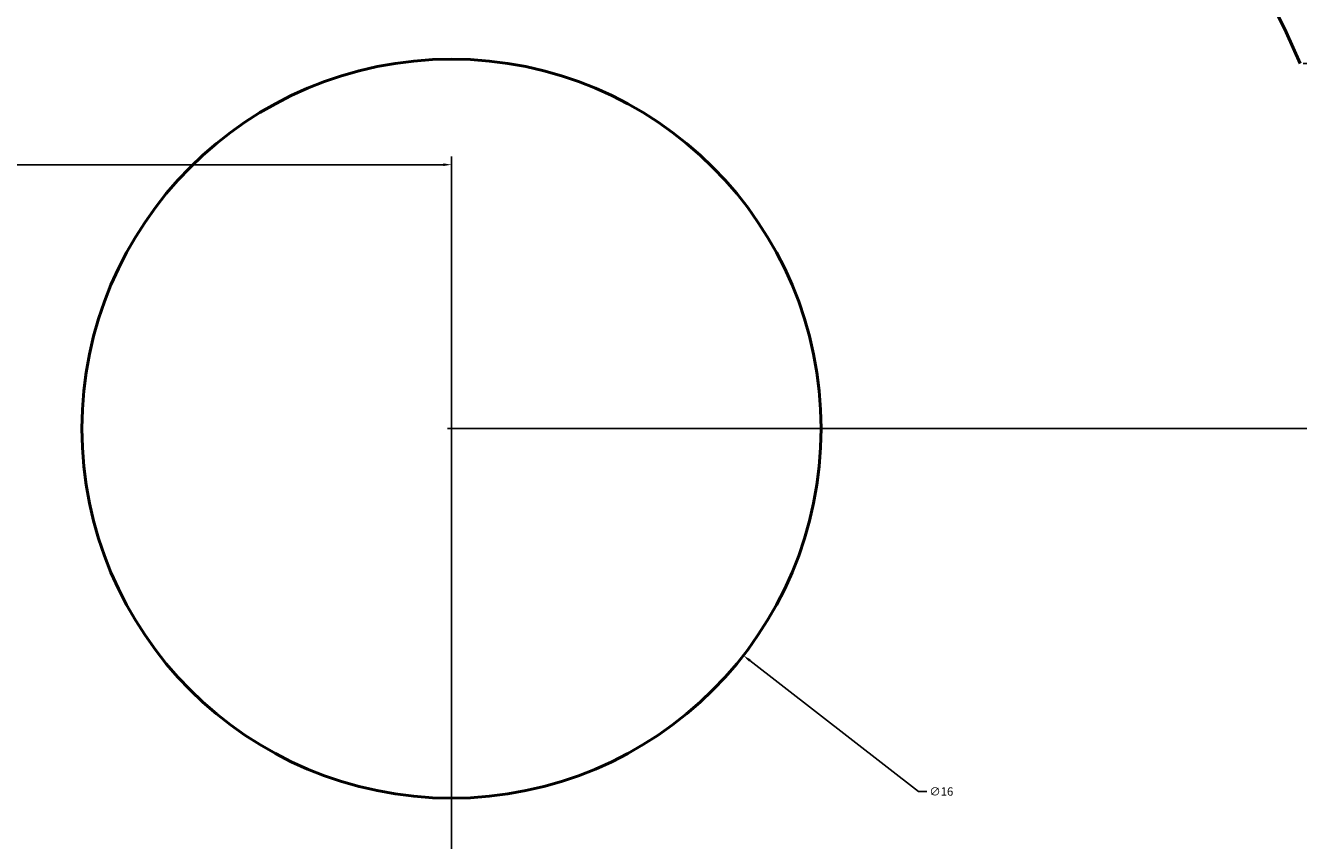
# Model space of a CAD drawing. Units: inches. Extents: x -14 to 108, y -9 to 83.
# Tile 9 of 13: x 38 to 65, y 28 to 46. Entities that reach past the tile are written whole.
import ezdxf

# ---------------------------------------------------------------- set-up
doc = ezdxf.new("R2010")
doc.units = ezdxf.units.IN
doc.header["$MEASUREMENT"] = 0
doc.layers.add('M-DIMS', color=2, linetype='Continuous', lineweight=18)
doc.layers.add('M-OUTL', color=7, linetype='Continuous', lineweight=50)
doc.styles.get("Standard").update_dxf_attribs({"font": 'arial.ttf'})
doc.dimstyles.get("Standard").update_dxf_attribs({"dimtxt": 0.18, "dimasz": 0.18, "dimexe": 0.18, "dimexo": 0.0625, "dimgap": 0.09, "dimtad": 0, "dimtih": 1, "dimtoh": 1, "dimzin": 0, "dimdsep": 46, "dimtxsty": 'Standard', "dimcen": 0.09, "dimadec": 0, "dimazin": 0, "dimtfac": 1, "dimtofl": 0, "dimtmove": 0, "dimatfit": 3, "dimfxl": 1, "dimtolj": 1, "dimtzin": 0, "dimarcsym": 0})

# ---------------------------------------------------------------- blocks, each defined once
blk = doc.blocks.new('*D7')
at = {"layer": 'Defpoints', "color": 0, "transparency": 16777216}
for p in [(47.098, 37.119), (5.951, 18.227), (47.098, -8.596)]:
    blk.add_point(p, dxfattribs=at)
at = {"layer": 'M-DIMS', "color": 0, "lineweight": -2, "transparency": 16777216}
for p, q in [((47.098, 37.057), (47.098, -8.776)), ((5.951, 18.165), (5.951, -8.776)), ((6.131, -8.596), (26.126, -8.596)), ((46.918, -8.596), (26.922, -8.596))]:
    blk.add_line(p, q, dxfattribs=at)
at = {"layer": 'M-DIMS', "color": 0, "transparency": 16777216}
for points in [[(6.131, -8.566), (6.131, -8.626), (5.951, -8.596)], [(46.918, -8.566), (46.918, -8.626), (47.098, -8.596)]]:
    blk.add_solid(points, dxfattribs=at)
at = {"layer": 'M-DIMS', "color": 0, "transparency": 16777216, "insert": (26.524, -8.596), "char_height": 0.18, "attachment_point": 5}
blk.add_mtext('\\A1;41.15', dxfattribs=at)
blk = doc.blocks.new('*D8')
at = {"layer": 'Defpoints', "color": 0, "transparency": 16777216}
for p in [(47.098, 37.119), (81.545, 18.227), (81.545, -8.596)]:
    blk.add_point(p, dxfattribs=at)
at = {"layer": 'M-DIMS', "color": 0, "lineweight": -2, "transparency": 16777216}
for p, q in [((47.098, 37.057), (47.098, -8.776)), ((81.545, 18.165), (81.545, -8.776)), ((47.278, -8.596), (63.927, -8.596)), ((81.365, -8.596), (64.716, -8.596))]:
    blk.add_line(p, q, dxfattribs=at)
at = {"layer": 'M-DIMS', "color": 0, "transparency": 16777216}
for points in [[(47.278, -8.566), (47.278, -8.626), (47.098, -8.596)], [(81.365, -8.566), (81.365, -8.626), (81.545, -8.596)]]:
    blk.add_solid(points, dxfattribs=at)
at = {"layer": 'M-DIMS', "color": 0, "transparency": 16777216, "insert": (64.321, -8.596), "char_height": 0.18, "attachment_point": 5}
blk.add_mtext('\\A1;34.45', dxfattribs=at)
blk = doc.blocks.new('*D11')
at = {"layer": 'Defpoints', "color": 0, "transparency": 16777216}
for p in [(47.098, 37.119), (107.813, 37.119), (86.478, 18.227)]:
    blk.add_point(p, dxfattribs=at)
at = {"layer": 'M-DIMS', "color": 0, "lineweight": -2, "transparency": 16777216}
for p, q in [((47.16, 37.119), (107.993, 37.119)), ((107.813, 36.939), (107.813, 27.855)), ((107.813, 18.407), (107.813, 27.491)), ((86.541, 18.227), (107.993, 18.227))]:
    blk.add_line(p, q, dxfattribs=at)
at = {"layer": 'M-DIMS', "color": 0, "transparency": 16777216}
for points in [[(107.783, 36.939), (107.843, 36.939), (107.813, 37.119)], [(107.783, 18.407), (107.843, 18.407), (107.813, 18.227)]]:
    blk.add_solid(points, dxfattribs=at)
at = {"layer": 'M-DIMS', "color": 0, "transparency": 16777216, "insert": (107.813, 27.673), "char_height": 0.18, "attachment_point": 5}
blk.add_mtext('\\A1;18.892', dxfattribs=at)
blk = doc.blocks.new('*D12')
at = {"layer": 'Defpoints', "color": 0, "transparency": 16777216}
for p in [(86.478, 57.664), (107.813, 57.664), (47.098, 37.119)]:
    blk.add_point(p, dxfattribs=at)
at = {"layer": 'M-DIMS', "color": 0, "lineweight": -2, "transparency": 16777216}
for p, q in [((86.541, 57.664), (107.993, 57.664)), ((107.813, 57.484), (107.813, 47.573)), ((107.813, 37.299), (107.813, 47.21)), ((47.16, 37.119), (107.993, 37.119))]:
    blk.add_line(p, q, dxfattribs=at)
at = {"layer": 'M-DIMS', "color": 0, "transparency": 16777216}
for points in [[(107.783, 57.484), (107.843, 57.484), (107.813, 57.664)], [(107.783, 37.299), (107.843, 37.299), (107.813, 37.119)]]:
    blk.add_solid(points, dxfattribs=at)
at = {"layer": 'M-DIMS', "color": 0, "transparency": 16777216, "insert": (107.813, 47.392), "char_height": 0.18, "attachment_point": 5}
blk.add_mtext('\\A1;20.544', dxfattribs=at)
blk = doc.blocks.new('*D14')
at = {"layer": 'Defpoints', "color": 0, "transparency": 16777216}
for p in [(47.098, 42.834), (16.928, 37.119), (47.098, 37.119)]:
    blk.add_point(p, dxfattribs=at)
at = {"layer": 'M-DIMS', "color": 0, "lineweight": -2, "transparency": 16777216}
for p, q in [((16.928, 37.182), (16.928, 43.014)), ((47.098, 37.182), (47.098, 43.014)), ((17.108, 42.834), (31.619, 42.834)), ((46.918, 42.834), (32.407, 42.834))]:
    blk.add_line(p, q, dxfattribs=at)
at = {"layer": 'M-DIMS', "color": 0, "transparency": 16777216}
for points in [[(17.108, 42.864), (17.108, 42.804), (16.928, 42.834)], [(46.918, 42.864), (46.918, 42.804), (47.098, 42.834)]]:
    blk.add_solid(points, dxfattribs=at)
at = {"layer": 'M-DIMS', "color": 0, "transparency": 16777216, "insert": (32.013, 42.834), "char_height": 0.18, "attachment_point": 5}
blk.add_mtext('\\A1;30.17', dxfattribs=at)
blk = doc.blocks.new('*D21')
at = {"layer": 'Defpoints', "color": 0, "transparency": 16777216}
for p in [(65.47, 45.024), (107.813, 45.024), (47.098, 37.119)]:
    blk.add_point(p, dxfattribs=at)
at = {"layer": 'M-DIMS', "color": 0, "lineweight": -2, "transparency": 16777216}
for p, q in [((65.532, 45.024), (107.993, 45.024)), ((107.813, 44.844), (107.813, 41.254)), ((107.813, 37.299), (107.813, 40.89)), ((47.16, 37.119), (107.993, 37.119))]:
    blk.add_line(p, q, dxfattribs=at)
at = {"layer": 'M-DIMS', "color": 0, "transparency": 16777216}
for points in [[(107.783, 44.844), (107.843, 44.844), (107.813, 45.024)], [(107.783, 37.299), (107.843, 37.299), (107.813, 37.119)]]:
    blk.add_solid(points, dxfattribs=at)
at = {"layer": 'M-DIMS', "color": 0, "transparency": 16777216, "insert": (107.813, 41.072), "char_height": 0.18, "attachment_point": 5}
blk.add_mtext('\\A1;7.905', dxfattribs=at)
blk = doc.blocks.new('*D28')
at = {"layer": 'Defpoints', "color": 0, "transparency": 16777216}
for p in [(40.782, 42.029), (53.414, 32.209)]:
    blk.add_point(p, dxfattribs=at)
at = {"layer": 'M-DIMS', "color": 0, "lineweight": -2, "transparency": 16777216}
for p, q in [((47.098, 37.029), (47.098, 37.209)), ((47.008, 37.119), (47.188, 37.119)), ((57.203, 29.263), (53.556, 32.099)), ((57.383, 29.263), (57.203, 29.263))]:
    blk.add_line(p, q, dxfattribs=at)
at = {"layer": 'M-DIMS', "color": 0, "transparency": 16777216}
blk.add_solid([(53.574, 32.122), (53.538, 32.075), (53.414, 32.209)], dxfattribs=at)
at = {"layer": 'M-DIMS', "color": 0, "transparency": 16777216, "insert": (57.7, 29.263), "char_height": 0.18, "attachment_point": 5}
blk.add_mtext('\\A1;∅16', dxfattribs=at)
blk = doc.blocks.new('*D30')
at = {"layer": 'Defpoints', "color": 0, "transparency": 16777216}
for p in [(59.745, 56.33), (47.098, 37.119)]:
    blk.add_point(p, dxfattribs=at)
at = {"layer": 'M-DIMS', "color": 0, "lineweight": -2, "transparency": 16777216}
for p, q in [((67.333, 67.856), (59.844, 56.48)), ((67.513, 67.856), (67.333, 67.856)), ((47.098, 37.029), (47.098, 37.209)), ((47.008, 37.119), (47.188, 37.119))]:
    blk.add_line(p, q, dxfattribs=at)
at = {"layer": 'M-DIMS', "color": 0, "transparency": 16777216}
blk.add_solid([(59.819, 56.497), (59.869, 56.464), (59.745, 56.33)], dxfattribs=at)
at = {"layer": 'M-DIMS', "color": 0, "transparency": 16777216, "insert": (67.818, 67.856), "char_height": 0.18, "attachment_point": 5}
blk.add_mtext('\\A1;R23', dxfattribs=at)
blk = doc.blocks.new('*D31')
at = {"layer": 'Defpoints', "color": 0, "transparency": 16777216}
for p in [(58.096, 53.824), (47.098, 37.119)]:
    blk.add_point(p, dxfattribs=at)
at = {"layer": 'M-DIMS', "color": 0, "lineweight": -2, "transparency": 16777216}
for p, q in [((64.695, 63.847), (58.195, 53.974)), ((64.875, 63.847), (64.695, 63.847)), ((47.098, 37.029), (47.098, 37.209)), ((47.008, 37.119), (47.188, 37.119))]:
    blk.add_line(p, q, dxfattribs=at)
at = {"layer": 'M-DIMS', "color": 0, "transparency": 16777216}
blk.add_solid([(58.17, 53.991), (58.22, 53.958), (58.096, 53.824)], dxfattribs=at)
at = {"layer": 'M-DIMS', "color": 0, "transparency": 16777216, "insert": (65.18, 63.847), "char_height": 0.18, "attachment_point": 5}
blk.add_mtext('\\A1;R20', dxfattribs=at)

msp = doc.modelspace()

# ---------------------------------------------------------------- linework, layer by layer
at = {"layer": 'M-OUTL'}
msp.add_circle((47.0979, 37.1193), 8, dxfattribs=at)
msp.add_arc((47.0979, 37.1193), 20, 23.2807, 90, dxfattribs=at)

# ---------------------------------------------------------------- dimensions: what is measured, and where the dimension line sits
at = {"layer": 'M-DIMS'}
for mpoint, picture, middle in [((59.745, 56.33), '*D30', (67.8183, 67.8564)), ((58.0959, 53.8239), '*D31', (65.1795, 63.8467))]:
    dim = msp.add_radius_dim(center=(47.0979, 37.1193), mpoint=mpoint, dimstyle='Standard', override={"dimdec": 0, "dimlfac": 1, "dimrnd": 0, "dimzin": 0, "dimdsep": 46, "dimlunit": 2}, dxfattribs=at)
    dim.commit()
    dim.dimension.update_dxf_attribs({"geometry": picture, "text_midpoint": middle, "dimtype": 164})
for base, p1, p2, angle, override, picture, middle in [((107.8129, 57.6637), (47.0979, 37.1193), (86.4784, 57.6637), 90, {"dimdec": 3, "dimlfac": 1, "dimrnd": 0, "dimzin": 0, "dimdsep": 46, "dimlunit": 2}, '*D12', (107.8129, 47.3915)), ((107.8129, 45.0241), (47.0979, 37.1193), (65.4695, 45.0241), 90, {"dimdec": 3, "dimlfac": 1, "dimrnd": 0, "dimzin": 0, "dimdsep": 46, "dimlunit": 2}, '*D21', (107.8129, 41.0717)), ((47.0979, 42.8343), (16.9278, 37.1193), (47.0979, 37.1193), 0, {"dimdec": 2, "dimlfac": 1, "dimrnd": 0, "dimzin": 0, "dimdsep": 46, "dimlunit": 2}, '*D14', (32.0129, 42.8343)), ((107.8129, 37.1193), (86.4784, 18.2274), (47.0979, 37.1193), 90, {"dimdec": 3, "dimlfac": 1, "dimrnd": 0, "dimzin": 0, "dimdsep": 46, "dimlunit": 2}, '*D11', (107.8129, 27.6733))]:
    dim = msp.add_linear_dim(base=base, p1=p1, p2=p2, angle=angle, dimstyle='Standard', override=override, dxfattribs=at)
    dim.commit()
    dim.dimension.update_dxf_attribs({"geometry": picture, "text_midpoint": middle})
dim = msp.add_diameter_dim_2p(p1=(40.782, 42.0294), p2=(53.4138, 32.2092), dimstyle='Standard', override={"dimdec": 0, "dimlfac": 1, "dimrnd": 0, "dimzin": 0, "dimdsep": 46, "dimlunit": 2}, dxfattribs=at)
dim.commit()
dim.dimension.update_dxf_attribs({"geometry": '*D28', "text_midpoint": (57.7002, 29.2632), "dimtype": 163})
for base, p1, p2, picture, middle in [((47.0979, -8.5957), (5.9508, 18.2274), (47.0979, 37.1193), '*D7', (26.5244, -8.5957)), ((81.5446, -8.5957), (47.0979, 37.1193), (81.5446, 18.2274), '*D8', (64.3213, -8.5957))]:
    dim = msp.add_linear_dim(base=base, p1=p1, p2=p2, dimstyle='Standard', override={"dimdec": 2, "dimlfac": 1, "dimrnd": 0, "dimzin": 0, "dimdsep": 46, "dimlunit": 2}, dxfattribs=at)
    dim.commit()
    dim.dimension.update_dxf_attribs({"geometry": picture, "text_midpoint": middle})

doc.saveas('drawing.dxf')
